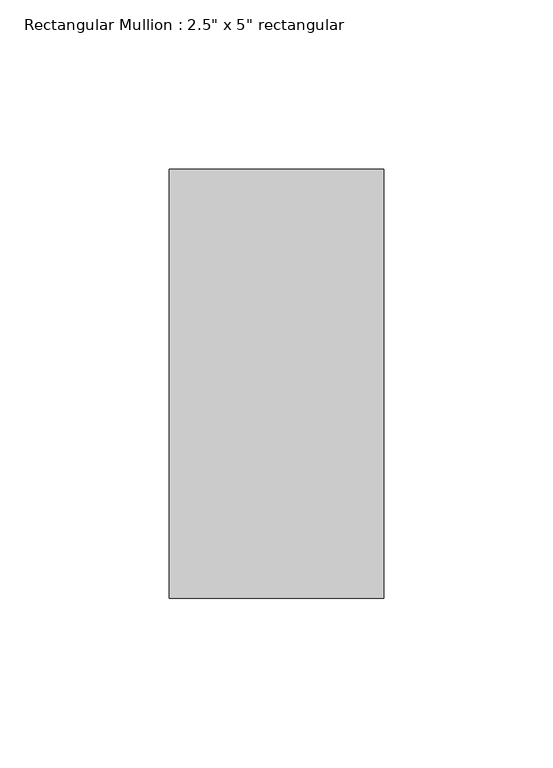
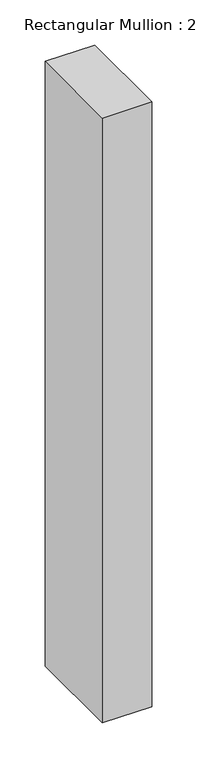
"""IFC4 building model written with IfcOpenShell, lengths in millimetres: member geometry."""

from ifc_helpers import new_model, si_unit, frame, origin, place, context, project, spatial, polyline, outline, extrude, source, transform, mapped, element, save


def member_c17f1be2(model_context):
    return source(origin(), model_context, "Body", "SweptSolid", [
        extrude(outline(polyline([(0.0, 63.5), (0.0, -63.5), (-63.5, -63.5), (-63.5, 63.5), (0.0, 63.5)])), frame((0.0, 0.0, -819.15), z_axis=(0.0, 0.0, 1.0), x_axis=(1.0, 0.0, 0.0)), (0.0, 0.0, 1.0), 819.15),
    ])


if __name__ == "__main__":
    model = new_model("IFC4")
    model_context = context("Model", 3, world=origin())
    ifc_project = project(units=[si_unit("LENGTHUNIT", "METRE", prefix="MILLI")], contexts=[model_context])
    site = spatial("IfcSite", under=ifc_project)
    building = spatial("IfcBuilding", under=site)
    placement = place(None, origin())
    member_shape = member_c17f1be2(model_context)
    element("IfcMember", 1, ObjectType="Rectangular Mullion : 2.5\" x 5\" rectangular", at=placement, inside=building, context=model_context, shape_type="MappedRepresentation", body=[
        mapped(member_shape, transform((0.0, 0.0, 0.0), x_axis=(1.0, 0.0, 0.0), y_axis=(0.0, 1.0, 0.0), z_axis=(0.0, 0.0, 1.0))),
    ])
    save(model, "model.ifc")

# Revit data of these elements
# Type "Rectangular Mullion : 2.5\" x 5\" rectangular"
#   built-in parameter 1007304 = 0.416667 (stored number, unit not read)
#   built-in parameter 1007301 = 0.104167 (stored number, unit not read)
#   built-in parameter 1007300 = 0.104167 (stored number, unit not read)
# Element 1 (IfcMember, "Rectangular Mullion : 2.5\" x 5\" rectangular")
#   Materials on its faces: "Aluminum"
# Materials
#   "Aluminum": class "Metal", colour RGB 247 247 247, transparency 0, Description = "Aluminum 6061", Cost = 0
